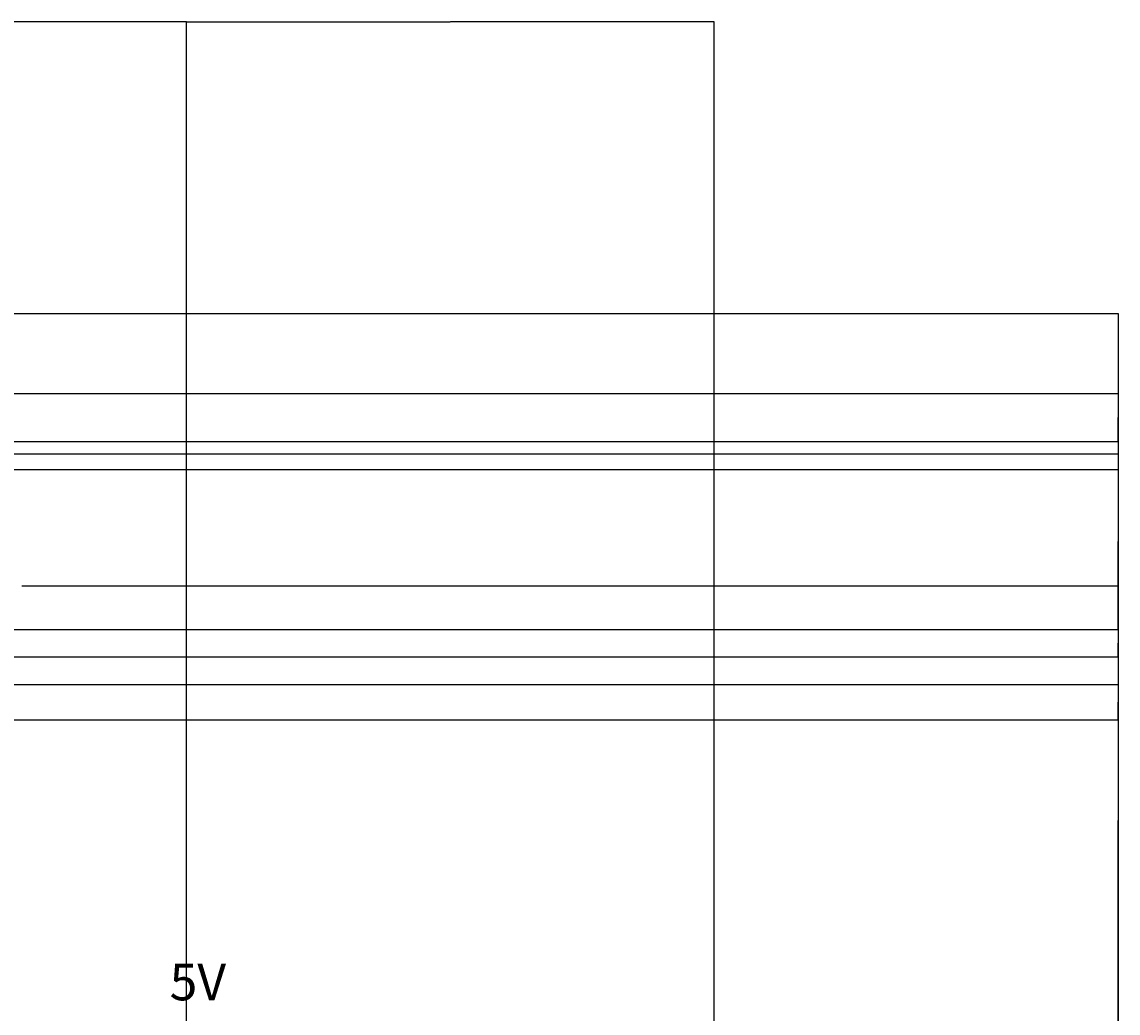
# Model space of a CAD drawing. Units: inches. Extents: x 35362 to 73946, y 43607 to 67532.
# Tile 134 of 134: x 67327 to 73946, y 61547 to 67532. Entities that reach past the tile are written whole.
import ezdxf

# ---------------------------------------------------------------- set-up
doc = ezdxf.new("R2010")
doc.units = ezdxf.units.IN
doc.header["$MEASUREMENT"] = 0
doc.layers.add('A-ANNO-DIMS', color=2, linetype='Continuous', lineweight=18)
doc.layers.add('E-ANNO-TEXT', color=5, linetype='Continuous', lineweight=18)
doc.styles.get("Standard").update_dxf_attribs({"font": 'arial.ttf'})
doc.dimstyles.get("Standard").update_dxf_attribs({"dimtxt": 0.18, "dimasz": 0.18, "dimexe": 0.18, "dimexo": 0.0625, "dimgap": 0.09, "dimtad": 0, "dimtih": 1, "dimtoh": 1, "dimdec": 4, "dimzin": 0, "dimdsep": 46, "dimtxsty": 'Standard', "dimcen": 0.09, "dimadec": 0, "dimazin": 0, "dimtfac": 1, "dimtdec": 4, "dimtofl": 0, "dimtmove": 0, "dimatfit": 3, "dimfxl": 1, "dimtolj": 1, "dimtzin": 0, "dimarcsym": 0})

# ---------------------------------------------------------------- blocks, each defined once
blk = doc.blocks.new('*D8')
at = {"layer": 'A-ANNO-DIMS', "color": 0, "lineweight": -2, "transparency": 16777216}
for p, q in [((66271.28651900003, 65771.51172800003), (73945.82566600003, 65771.51172800003)), ((73945.64566600005, 65771.33172800003), (73945.64566600005, 59737.03093663782)), ((73945.64566600005, 53702.36633900002), (73945.64566600005, 59736.66713036224)), ((72185.70816600003, 53702.18633900003), (73945.82566600003, 53702.18633900003))]:
    blk.add_line(p, q, dxfattribs=at)
at = {"layer": 'A-ANNO-DIMS', "color": 0, "transparency": 16777216}
for points in [[(73945.61566600006, 65771.33172800003), (73945.67566600005, 65771.33172800003), (73945.64566600005, 65771.51172800003)], [(73945.61566600006, 53702.36633900002), (73945.67566600005, 53702.36633900002), (73945.64566600005, 53702.18633900003)]]:
    blk.add_solid(points, dxfattribs=at)
at = {"layer": 'Defpoints', "color": 0, "transparency": 16777216}
for p in [(66271.22401900003, 65771.51172800003), (73945.64566600005, 65771.51172800003), (72185.64566600003, 53702.18633900003)]:
    blk.add_point(p, dxfattribs=at)
at = {"layer": 'A-ANNO-DIMS', "color": 0, "transparency": 16777216, "insert": (73945.64566600005, 59736.84903349999), "char_height": 0.18, "attachment_point": 5}
blk.add_mtext('\\A1;12069', dxfattribs=at)
blk = doc.blocks.new('*D35')
at = {"layer": 'A-ANNO-DIMS', "color": 0, "lineweight": -2, "transparency": 16777216}
for p, q in [((61240.907336, 59185.206457), (61240.907336, 67531.691728)), ((61241.08733599999, 67531.51172799998), (64780.42646373397, 67531.51172799998)), ((68320.69076200001, 67531.51172799998), (64781.35163426603, 67531.51172799998)), ((68320.870762, 60122.408832), (68320.870762, 67531.691728))]:
    blk.add_line(p, q, dxfattribs=at)
at = {"layer": 'A-ANNO-DIMS', "color": 0, "transparency": 16777216}
for points in [[(61241.08733599999, 67531.541728), (61241.08733599999, 67531.481728), (61240.907336, 67531.51172799998)], [(68320.69076200001, 67531.541728), (68320.69076200001, 67531.481728), (68320.870762, 67531.51172799998)]]:
    blk.add_solid(points, dxfattribs=at)
at = {"layer": 'Defpoints', "color": 0, "transparency": 16777216}
for p in [(68320.870762, 67531.51172799998), (68320.870762, 60122.346332), (61240.907336, 59185.14395699999)]:
    blk.add_point(p, dxfattribs=at)
at = {"layer": 'A-ANNO-DIMS', "color": 0, "transparency": 16777216, "insert": (64780.889049, 67531.51172799998), "char_height": 0.18, "attachment_point": 5}
blk.add_mtext('\\A1;7080.0', dxfattribs=at)
blk = doc.blocks.new('*D66')
at = {"layer": 'A-ANNO-DIMS', "color": 0, "lineweight": -2, "transparency": 16777216}
for p, q in [((67326.70224100004, 64127.44160800003), (73945.82566600003, 64127.44160800003)), ((73945.64566600005, 64127.26160800003), (73945.64566600005, 62710.54579452936)), ((73945.64566600005, 61293.46605200003), (73945.64566600005, 62710.1818654707)), ((67326.70224100004, 61293.28605200003), (73945.82566600003, 61293.28605200003))]:
    blk.add_line(p, q, dxfattribs=at)
at = {"layer": 'A-ANNO-DIMS', "color": 0, "transparency": 16777216}
for points in [[(73945.61566600006, 64127.26160800003), (73945.67566600005, 64127.26160800003), (73945.64566600005, 64127.44160800003)], [(73945.61566600006, 61293.46605200003), (73945.67566600005, 61293.46605200003), (73945.64566600005, 61293.28605200003)]]:
    blk.add_solid(points, dxfattribs=at)
at = {"layer": 'Defpoints', "color": 0, "transparency": 16777216}
for p in [(67326.63974100004, 64127.44160800003), (73945.64566600005, 64127.44160800003), (67326.63974100004, 61293.28605200003)]:
    blk.add_point(p, dxfattribs=at)
at = {"layer": 'A-ANNO-DIMS', "color": 0, "transparency": 16777216, "insert": (73945.64566600005, 62710.36383), "char_height": 0.18, "attachment_point": 5}
blk.add_mtext('\\A1;2834.2', dxfattribs=at)
blk = doc.blocks.new('*D69')
at = {"layer": 'A-ANNO-DIMS', "color": 0, "lineweight": -2, "transparency": 16777216}
for p, q in [((68320.870762, 60122.408832), (68320.870762, 67531.691728)), ((68321.050762, 67531.51172799998), (69913.30289879469, 67531.51172799998)), ((71506.482539, 67531.51172799998), (69914.23040220531, 67531.51172799998)), ((71506.662539, 59451.647447), (71506.662539, 67531.691728))]:
    blk.add_line(p, q, dxfattribs=at)
at = {"layer": 'A-ANNO-DIMS', "color": 0, "transparency": 16777216}
for points in [[(68321.050762, 67531.541728), (68321.050762, 67531.481728), (68320.870762, 67531.51172799998)], [(71506.482539, 67531.541728), (71506.482539, 67531.481728), (71506.662539, 67531.51172799998)]]:
    blk.add_solid(points, dxfattribs=at)
at = {"layer": 'Defpoints', "color": 0, "transparency": 16777216}
for p in [(71506.662539, 67531.51172799998), (68320.870762, 60122.346332), (71506.662539, 59451.584947)]:
    blk.add_point(p, dxfattribs=at)
at = {"layer": 'A-ANNO-DIMS', "color": 0, "transparency": 16777216, "insert": (69913.76665050001, 67531.51172799998), "char_height": 0.18, "attachment_point": 5}
blk.add_mtext('\\A1;3185.8', dxfattribs=at)
blk = doc.blocks.new('*D70')
at = {"layer": 'A-ANNO-DIMS', "color": 0, "lineweight": -2, "transparency": 16777216}
for p, q in [((60785.27513900002, 64923.75242000003), (73945.82566600003, 64923.75242000003)), ((73945.64566600005, 64923.57242000003), (73945.64566600005, 62054.63015302935)), ((73945.64566600005, 59185.32395700003), (73945.64566600005, 62054.26622397069)), ((61240.96983600002, 59185.14395700003), (73945.82566600003, 59185.14395700003))]:
    blk.add_line(p, q, dxfattribs=at)
at = {"layer": 'A-ANNO-DIMS', "color": 0, "transparency": 16777216}
for points in [[(73945.61566600006, 64923.57242000003), (73945.67566600005, 64923.57242000003), (73945.64566600005, 64923.75242000003)], [(73945.61566600006, 59185.32395700003), (73945.67566600005, 59185.32395700003), (73945.64566600005, 59185.14395700003)]]:
    blk.add_solid(points, dxfattribs=at)
at = {"layer": 'Defpoints', "color": 0, "transparency": 16777216}
for p in [(60785.21263900002, 64923.75242000003), (73945.64566600005, 64923.75242000003), (61240.90733600002, 59185.14395700003)]:
    blk.add_point(p, dxfattribs=at)
at = {"layer": 'A-ANNO-DIMS', "color": 0, "transparency": 16777216, "insert": (73945.64566600005, 62054.44818849999), "char_height": 0.18, "attachment_point": 5}
blk.add_mtext('\\A1;5738.6', dxfattribs=at)
blk = doc.blocks.new('*D71')
at = {"layer": 'A-ANNO-DIMS', "color": 0, "lineweight": -2, "transparency": 16777216}
for p, q in [((63159.24181700003, 64828.55626700002), (73945.82566600003, 64828.55626700002)), ((73945.64566600005, 64828.37626700002), (73945.64566600005, 62007.03207652936)), ((73945.64566600005, 59185.32395700003), (73945.64566600005, 62006.6681474707)), ((61240.96983600002, 59185.14395700003), (73945.82566600003, 59185.14395700003))]:
    blk.add_line(p, q, dxfattribs=at)
at = {"layer": 'A-ANNO-DIMS', "color": 0, "transparency": 16777216}
for points in [[(73945.61566600006, 64828.37626700002), (73945.67566600005, 64828.37626700002), (73945.64566600005, 64828.55626700002)], [(73945.61566600006, 59185.32395700003), (73945.67566600005, 59185.32395700003), (73945.64566600005, 59185.14395700003)]]:
    blk.add_solid(points, dxfattribs=at)
at = {"layer": 'Defpoints', "color": 0, "transparency": 16777216}
for p in [(63159.17931700003, 64828.55626700002), (73945.64566600005, 64828.55626700002), (61240.90733600002, 59185.14395700003)]:
    blk.add_point(p, dxfattribs=at)
at = {"layer": 'A-ANNO-DIMS', "color": 0, "transparency": 16777216, "insert": (73945.64566600005, 62006.85011199999), "char_height": 0.18, "attachment_point": 5}
blk.add_mtext('\\A1;5643.4', dxfattribs=at)
blk = doc.blocks.new('*D97')
at = {"layer": 'A-ANNO-DIMS', "color": 0, "lineweight": -2, "transparency": 16777216}
for p, q in [((53988.67814800002, 65288.88854300003), (73945.82566600003, 65288.88854300003)), ((73945.64566600005, 65288.70854300003), (73945.64566600005, 65143.46751513782)), ((73945.64566600005, 64997.86268100002), (73945.64566600005, 65143.10370886223)), ((53988.67814800002, 64997.68268100003), (73945.82566600003, 64997.68268100003))]:
    blk.add_line(p, q, dxfattribs=at)
at = {"layer": 'A-ANNO-DIMS', "color": 0, "transparency": 16777216}
for points in [[(73945.61566600006, 65288.70854300003), (73945.67566600005, 65288.70854300003), (73945.64566600005, 65288.88854300003)], [(73945.61566600006, 64997.86268100002), (73945.67566600005, 64997.86268100002), (73945.64566600005, 64997.68268100003)]]:
    blk.add_solid(points, dxfattribs=at)
at = {"layer": 'Defpoints', "color": 0, "transparency": 16777216}
for p in [(53988.61564800003, 65288.88854300003), (73945.64566600005, 65288.88854300003), (53988.61564800003, 64997.68268100003)]:
    blk.add_point(p, dxfattribs=at)
at = {"layer": 'A-ANNO-DIMS', "color": 0, "transparency": 16777216, "insert": (73945.64566600005, 65143.28561199999), "char_height": 0.18, "attachment_point": 5}
blk.add_mtext('\\A1;291.2', dxfattribs=at)
blk = doc.blocks.new('*D103')
at = {"layer": 'A-ANNO-DIMS', "color": 0, "lineweight": -2, "transparency": 16777216}
for p, q in [((56172.14479300002, 63863.49026700003), (73945.82566600003, 63863.49026700003)), ((73945.64566600005, 63863.31026700003), (73945.64566600005, 63780.36050313782)), ((73945.64566600005, 63697.04693300002), (73945.64566600005, 63779.99669686224)), ((56272.53121400003, 63696.86693300002), (73945.82566600003, 63696.86693300002))]:
    blk.add_line(p, q, dxfattribs=at)
at = {"layer": 'A-ANNO-DIMS', "color": 0, "transparency": 16777216}
for points in [[(73945.61566600006, 63863.31026700003), (73945.67566600005, 63863.31026700003), (73945.64566600005, 63863.49026700003)], [(73945.61566600006, 63697.04693300002), (73945.67566600005, 63697.04693300002), (73945.64566600005, 63696.86693300002)]]:
    blk.add_solid(points, dxfattribs=at)
at = {"layer": 'Defpoints', "color": 0, "transparency": 16777216}
for p in [(56172.08229300002, 63863.49026700003), (73945.64566600005, 63863.49026700003), (56272.46871400003, 63696.86693300002)]:
    blk.add_point(p, dxfattribs=at)
at = {"layer": 'A-ANNO-DIMS', "color": 0, "transparency": 16777216, "insert": (73945.64566600005, 63780.17859999999), "char_height": 0.18, "attachment_point": 5}
blk.add_mtext('\\A1;166.62', dxfattribs=at)
blk = doc.blocks.new('*D105')
at = {"layer": 'A-ANNO-DIMS', "color": 0, "lineweight": -2, "transparency": 16777216}
for p, q in [((56223.01523600002, 63531.49645700002), (73945.82566600003, 63531.49645700002)), ((73945.64566600005, 63531.31645700003), (73945.64566600005, 63424.99614102936)), ((73945.64566600005, 63318.31189600003), (73945.64566600005, 63424.6322119707)), ((56223.01523600002, 63318.13189600002), (73945.82566600003, 63318.13189600002))]:
    blk.add_line(p, q, dxfattribs=at)
at = {"layer": 'A-ANNO-DIMS', "color": 0, "transparency": 16777216}
for points in [[(73945.61566600006, 63531.31645700003), (73945.67566600005, 63531.31645700003), (73945.64566600005, 63531.49645700002)], [(73945.61566600006, 63318.31189600003), (73945.67566600005, 63318.31189600003), (73945.64566600005, 63318.13189600002)]]:
    blk.add_solid(points, dxfattribs=at)
at = {"layer": 'Defpoints', "color": 0, "transparency": 16777216}
for p in [(56222.95273600003, 63531.49645700002), (73945.64566600005, 63531.49645700002), (56222.95273600003, 63318.13189600002)]:
    blk.add_point(p, dxfattribs=at)
at = {"layer": 'A-ANNO-DIMS', "color": 0, "transparency": 16777216, "insert": (73945.64566600005, 63424.8141765), "char_height": 0.18, "attachment_point": 5}
blk.add_mtext('\\A1;213.36', dxfattribs=at)
blk = doc.blocks.new('*D106')
at = {"layer": 'A-ANNO-DIMS', "color": 0, "lineweight": -2, "transparency": 16777216}
for p, q in [((56464.79693200002, 64923.75242000003), (73945.82566600003, 64923.75242000003)), ((73945.64566600005, 64923.57242000003), (73945.64566600005, 64393.80330802936)), ((73945.64566600005, 63863.67026700003), (73945.64566600005, 64393.4393789707)), ((56172.14479300002, 63863.49026700003), (73945.82566600003, 63863.49026700003))]:
    blk.add_line(p, q, dxfattribs=at)
at = {"layer": 'A-ANNO-DIMS', "color": 0, "transparency": 16777216}
for points in [[(73945.61566600006, 64923.57242000003), (73945.67566600005, 64923.57242000003), (73945.64566600005, 64923.75242000003)], [(73945.61566600006, 63863.67026700003), (73945.67566600005, 63863.67026700003), (73945.64566600005, 63863.49026700003)]]:
    blk.add_solid(points, dxfattribs=at)
at = {"layer": 'Defpoints', "color": 0, "transparency": 16777216}
for p in [(56464.73443200003, 64923.75242000003), (56172.08229300002, 63863.49026700003), (73945.64566600005, 63863.49026700003)]:
    blk.add_point(p, dxfattribs=at)
at = {"layer": 'A-ANNO-DIMS', "color": 0, "transparency": 16777216, "insert": (73945.64566600005, 64393.62134349998), "char_height": 0.18, "attachment_point": 5}
blk.add_mtext('\\A1;1060.3', dxfattribs=at)

msp = doc.modelspace()

# ---------------------------------------------------------------- texts
at = {"layer": 'E-ANNO-TEXT'}
msp.add_text('5V', height=220.8659825270206, dxfattribs=at).set_placement((68218.68602242187, 61623.74931593589))

# ---------------------------------------------------------------- dimensions: what is measured, and where the dimension line sits
at = {"layer": 'A-ANNO-DIMS'}
for base, p1, p2, picture, middle in [((68320.870762, 67531.51172799998), (61240.907336, 59185.14395699999), (68320.870762, 60122.346332), '*D35', (64780.889049, 67531.51172799998)), ((71506.662539, 67531.51172799998), (68320.870762, 60122.346332), (71506.662539, 59451.584947), '*D69', (69913.76665050001, 67531.51172799998))]:
    dim = msp.add_linear_dim(base=base, p1=p1, p2=p2, dimstyle='Standard', override={"dimdec": 1, "dimlfac": 1, "dimrnd": 0, "dimzin": 0, "dimdsep": 46, "dimlunit": 2}, dxfattribs=at)
    dim.commit()
    dim.dimension.update_dxf_attribs({"geometry": picture, "text_midpoint": middle})
for base, p1, p2, override, picture, middle in [((73945.64566600005, 65771.51172800003), (72185.645666, 53702.186339), (66271.224019, 65771.51172799998), {"dimdec": 0, "dimlfac": 1, "dimrnd": 0, "dimzin": 0, "dimdsep": 46, "dimlunit": 2}, '*D8', (73945.64566600005, 59736.84903349999)), ((73945.64566600005, 65288.88854300003), (53988.61564799999, 64997.682681), (53988.61564799999, 65288.888543), {"dimdec": 1, "dimlfac": 1, "dimrnd": 0, "dimzin": 0, "dimdsep": 46, "dimlunit": 2}, '*D97', (73945.64566600005, 65143.28561199999)), ((73945.64566600005, 63863.49026700003), (56464.73443199999, 64923.75241999999), (56172.082293, 63863.490267), {"dimdec": 1, "dimlfac": 1, "dimrnd": 0, "dimzin": 0, "dimdsep": 46, "dimlunit": 2}, '*D106', (73945.64566600005, 64393.62134349998)), ((73945.64566600005, 64923.75242000003), (61240.907336, 59185.14395699999), (60785.21263899999, 64923.75241999999), {"dimdec": 1, "dimlfac": 1, "dimrnd": 0, "dimzin": 0, "dimdsep": 46, "dimlunit": 2}, '*D70', (73945.64566600005, 62054.44818849999)), ((73945.64566600005, 64828.55626700002), (61240.907336, 59185.14395699999), (63159.179317, 64828.556267), {"dimdec": 1, "dimlfac": 1, "dimrnd": 0, "dimzin": 0, "dimdsep": 46, "dimlunit": 2}, '*D71', (73945.64566600005, 62006.85011199999)), ((73945.64566600005, 64127.44160800003), (67326.639741, 61293.286052), (67326.639741, 64127.44160799999), {"dimdec": 1, "dimlfac": 1, "dimrnd": 0, "dimzin": 0, "dimdsep": 46, "dimlunit": 2}, '*D66', (73945.64566600005, 62710.36383)), ((73945.64566600005, 63863.49026700003), (56272.468714, 63696.866933), (56172.082293, 63863.490267), {"dimdec": 2, "dimlfac": 1, "dimrnd": 0, "dimzin": 0, "dimdsep": 46, "dimlunit": 2}, '*D103', (73945.64566600005, 63780.17859999999)), ((73945.64566600005, 63531.49645700002), (56222.95273599999, 63318.131896), (56222.95273599999, 63531.496457), {"dimdec": 2, "dimlfac": 1, "dimrnd": 0, "dimzin": 0, "dimdsep": 46, "dimlunit": 2}, '*D105', (73945.64566600005, 63424.8141765))]:
    dim = msp.add_linear_dim(base=base, p1=p1, p2=p2, angle=90, dimstyle='Standard', override=override, dxfattribs=at)
    dim.commit()
    dim.dimension.update_dxf_attribs({"geometry": picture, "text_midpoint": middle})

doc.saveas('drawing.dxf')
